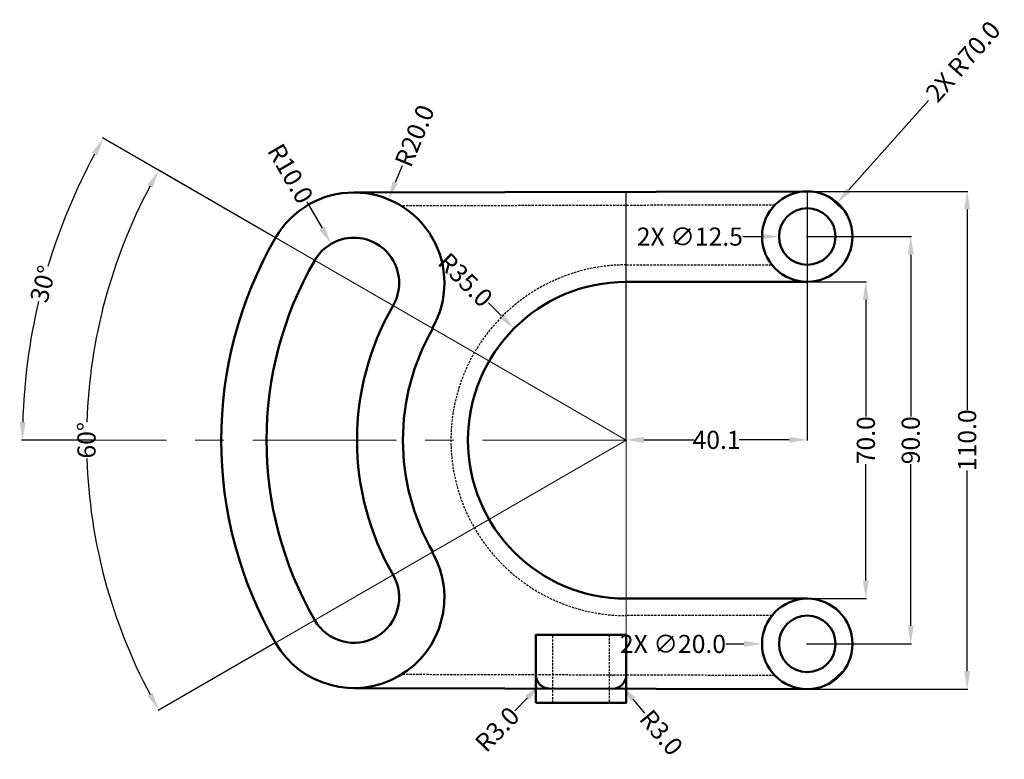
# Model space of a CAD drawing. Units: millimetres. Extents: x 1081 to 1299, y 820 to 983.
import ezdxf

# ---------------------------------------------------------------- set-up
doc = ezdxf.new("R2010")
doc.units = ezdxf.units.MM
doc.header["$MEASUREMENT"] = 0
doc.linetypes.add('CENTER', pattern=[50.8, 31.75, -6.35, 6.35, -6.35])
doc.linetypes.add('HIDDENX2', pattern=[0.75, 0.5, -0.25])
for name, color, linetype, lineweight in [('M-CNTR', 4, 'CENTER', 18), ('M-CONS', 8, 'Continuous', 13), ('M-DIMS', 2, 'Continuous', 25), ('M-HIDN', 3, 'HIDDENX2', 25), ('M-OUTL', 7, 'Continuous', 50)]:
    doc.layers.add(name, color=color, linetype=linetype, lineweight=lineweight)
doc.styles.get("Standard").update_dxf_attribs({"font": 'arial.ttf'})
doc.dimstyles.get("Standard").update_dxf_attribs({"dimtxt": 4, "dimasz": 4, "dimexe": 0.18, "dimexo": 0.0625, "dimgap": 0.09, "dimtad": 0, "dimdec": 1, "dimzin": 0, "dimdsep": 46, "dimtxsty": 'Standard', "dimcen": 0.09, "dimadec": 0, "dimazin": 0, "dimtfac": 1, "dimtdec": 1, "dimtofl": 0, "dimtmove": 0, "dimatfit": 3, "dimfxl": 1, "dimtolj": 1, "dimtzin": 0, "dimarcsym": 0})

# ---------------------------------------------------------------- blocks, each defined once
blk = doc.blocks.new('*D1')
at = {"layer": 'Defpoints', "color": 0, "transparency": 16777216}
for p in [(1137.47, 935.11), (1097.95, 910.82), (1215.42, 890.11), (1215.42, 890.11), (1137.91, 845.36)]:
    blk.add_point(p, dxfattribs=at)
at = {"layer": 'M-DIMS', "color": 0, "lineweight": -2, "transparency": 16777216}
for p, q in [((1137.42, 935.14), (1111.96, 949.84)), ((1137.85, 845.33), (1111.96, 830.38))]:
    blk.add_line(p, q, dxfattribs=at)
for start, end in [(151.9215, 178.0664), (181.9336, 208.0785)]:
    blk.add_arc((1215.42, 890.11), 119.28, start, end, dxfattribs=at)
at = {"layer": 'M-DIMS', "color": 0, "transparency": 16777216}
for points in [[(1109.59, 946.57), (1110.76, 945.93), (1112.12, 949.75)], [(1110.76, 834.29), (1109.59, 833.64), (1112.12, 830.47)]]:
    blk.add_solid(points, dxfattribs=at)
at = {"layer": 'M-DIMS', "color": 0, "transparency": 16777216, "insert": (1096.14, 890.11), "char_height": 4, "attachment_point": 5, "rotation": 90}
blk.add_mtext('\\A1;60°', dxfattribs=at)
blk = doc.blocks.new('*D2')
at = {"layer": 'Defpoints', "color": 0, "transparency": 16777216}
for p in [(1090.03, 935.75), (1137.47, 935.11), (1098.27, 890.11), (1215.42, 890.11), (1215.42, 890.11)]:
    blk.add_point(p, dxfattribs=at)
at = {"layer": 'M-DIMS', "color": 0, "lineweight": -2, "transparency": 16777216}
for p, q in [((1137.42, 935.14), (1099.7, 956.92)), ((1098.21, 890.11), (1081.8, 890.11))]:
    blk.add_line(p, q, dxfattribs=at)
for start, end in [(151.7176, 163.2769), (166.7231, 178.2824)]:
    blk.add_arc((1215.42, 890.11), 133.44, start, end, dxfattribs=at)
at = {"layer": 'M-DIMS', "color": 0, "transparency": 16777216}
for points in [[(1097.33, 953.66), (1098.49, 953.01), (1099.86, 956.83)], [(1082.71, 894.1), (1081.38, 894.12), (1081.98, 890.11)]]:
    blk.add_solid(points, dxfattribs=at)
at = {"layer": 'M-DIMS', "color": 0, "transparency": 16777216, "insert": (1086.53, 924.64), "char_height": 4, "attachment_point": 5, "rotation": 75}
blk.add_mtext('\\A1;30°', dxfattribs=at)
blk = doc.blocks.new('*D3')
at = {"layer": 'Defpoints', "color": 0, "transparency": 16777216}
for p in [(1190.64, 914.82), (1215.42, 890.11)]:
    blk.add_point(p, dxfattribs=at)
at = {"layer": 'M-DIMS', "color": 0, "lineweight": -2, "transparency": 16777216}
for p, q in [((1184.97, 920.47), (1187.8, 917.65)), ((1215.33, 890.11), (1215.51, 890.11)), ((1215.42, 890.02), (1215.42, 890.2))]:
    blk.add_line(p, q, dxfattribs=at)
at = {"layer": 'M-DIMS', "color": 0, "transparency": 16777216}
blk.add_solid([(1188.27, 918.12), (1187.33, 917.18), (1190.64, 914.82)], dxfattribs=at)
at = {"layer": 'M-DIMS', "color": 0, "transparency": 16777216, "insert": (1179.88, 925.55), "char_height": 4, "attachment_point": 5, "rotation": 315.0772}
blk.add_mtext('\\A1;R35.0', dxfattribs=at)
blk = doc.blocks.new('*D4')
at = {"layer": 'Defpoints', "color": 0, "transparency": 16777216}
for p in [(1162.85, 943.35), (1155.23, 924.86)]:
    blk.add_point(p, dxfattribs=at)
at = {"layer": 'M-DIMS', "color": 0, "lineweight": -2, "transparency": 16777216}
for p, q in [((1165.9, 950.74), (1164.38, 947.05)), ((1155.14, 924.86), (1155.32, 924.86)), ((1155.23, 924.77), (1155.23, 924.95))]:
    blk.add_line(p, q, dxfattribs=at)
at = {"layer": 'M-DIMS', "color": 0, "transparency": 16777216}
blk.add_solid([(1163.76, 947.3), (1164.99, 946.79), (1162.85, 943.35)], dxfattribs=at)
at = {"layer": 'M-DIMS', "color": 0, "transparency": 16777216, "insert": (1168.64, 957.39), "char_height": 4, "attachment_point": 5, "rotation": 67.5926}
blk.add_mtext('\\A1;R20.0', dxfattribs=at)
blk = doc.blocks.new('*D5')
at = {"layer": 'Defpoints', "color": 0, "transparency": 16777216}
for p in [(1150.21, 933.51), (1155.23, 924.86)]:
    blk.add_point(p, dxfattribs=at)
at = {"layer": 'M-DIMS', "color": 0, "lineweight": -2, "transparency": 16777216}
for p, q in [((1144.82, 942.8), (1148.2, 936.97)), ((1155.14, 924.86), (1155.32, 924.86)), ((1155.23, 924.77), (1155.23, 924.95))]:
    blk.add_line(p, q, dxfattribs=at)
at = {"layer": 'M-DIMS', "color": 0, "transparency": 16777216}
blk.add_solid([(1148.78, 937.3), (1147.63, 936.63), (1150.21, 933.51)], dxfattribs=at)
at = {"layer": 'M-DIMS', "color": 0, "transparency": 16777216, "insert": (1141.21, 949.03), "char_height": 4, "attachment_point": 5, "rotation": 300.1178}
blk.add_mtext('\\A1;R10.0', dxfattribs=at)
blk = doc.blocks.new('*D6')
at = {"layer": 'Defpoints', "color": 0, "transparency": 16777216}
for p in [(1212.42, 838.22), (1214.36, 835.93)]:
    blk.add_point(p, dxfattribs=at)
at = {"layer": 'M-DIMS', "color": 0, "lineweight": -2, "transparency": 16777216}
for p, q in [((1212.33, 838.22), (1212.51, 838.22)), ((1212.42, 838.13), (1212.42, 838.31)), ((1219.53, 829.82), (1216.94, 832.87))]:
    blk.add_line(p, q, dxfattribs=at)
at = {"layer": 'M-DIMS', "color": 0, "transparency": 16777216}
blk.add_solid([(1217.45, 833.31), (1216.43, 832.44), (1214.36, 835.93)], dxfattribs=at)
at = {"layer": 'M-DIMS', "color": 0, "transparency": 16777216, "insert": (1223.17, 825.52), "char_height": 4, "attachment_point": 5, "rotation": 310.2705}
blk.add_mtext('\\A1;R3.0', dxfattribs=at)
blk = doc.blocks.new('*D7')
at = {"layer": 'Defpoints', "color": 0, "transparency": 16777216}
for p in [(1198.42, 838.25), (1196.34, 836.09)]:
    blk.add_point(p, dxfattribs=at)
at = {"layer": 'M-DIMS', "color": 0, "lineweight": -2, "transparency": 16777216}
for p, q in [((1198.33, 838.25), (1198.51, 838.25)), ((1198.42, 838.16), (1198.42, 838.34)), ((1190.8, 830.31), (1193.57, 833.2))]:
    blk.add_line(p, q, dxfattribs=at)
at = {"layer": 'M-DIMS', "color": 0, "transparency": 16777216}
blk.add_solid([(1193.09, 833.66), (1194.05, 832.74), (1196.34, 836.09)], dxfattribs=at)
at = {"layer": 'M-DIMS', "color": 0, "transparency": 16777216, "insert": (1186.9, 826.24), "char_height": 4, "attachment_point": 5, "rotation": 46.199}
blk.add_mtext('\\A1;R3.0', dxfattribs=at)
blk = doc.blocks.new('*D8')
at = {"layer": 'Defpoints', "color": 0, "transparency": 16777216}
for p in [(1255.42, 935.11), (1255.42, 845.11), (1278.28, 845.11)]:
    blk.add_point(p, dxfattribs=at)
at = {"layer": 'M-DIMS', "color": 0, "lineweight": -2, "transparency": 16777216}
for p, q in [((1255.48, 935.11), (1278.46, 935.11)), ((1278.28, 931.11), (1278.28, 895.39)), ((1278.28, 849.11), (1278.28, 884.83)), ((1255.48, 845.11), (1278.46, 845.11))]:
    blk.add_line(p, q, dxfattribs=at)
at = {"layer": 'M-DIMS', "color": 0, "transparency": 16777216}
for points in [[(1277.61, 931.11), (1278.95, 931.11), (1278.28, 935.11)], [(1277.61, 849.11), (1278.95, 849.11), (1278.28, 845.11)]]:
    blk.add_solid(points, dxfattribs=at)
at = {"layer": 'M-DIMS', "color": 0, "transparency": 16777216, "insert": (1278.28, 890.11), "char_height": 4, "attachment_point": 5, "rotation": 90}
blk.add_mtext('\\A1;90.0', dxfattribs=at)
blk = doc.blocks.new('*D9')
at = {"layer": 'Defpoints', "color": 0, "transparency": 16777216}
for p in [(1255.42, 945.11), (1290.74, 945.11), (1255.42, 835.11)]:
    blk.add_point(p, dxfattribs=at)
at = {"layer": 'M-DIMS', "color": 0, "lineweight": -2, "transparency": 16777216}
for p, q in [((1255.48, 945.11), (1290.92, 945.11)), ((1290.74, 941.11), (1290.74, 896.75)), ((1290.74, 839.11), (1290.74, 883.46)), ((1255.48, 835.11), (1290.92, 835.11))]:
    blk.add_line(p, q, dxfattribs=at)
at = {"layer": 'M-DIMS', "color": 0, "transparency": 16777216}
for points in [[(1290.07, 941.11), (1291.4, 941.11), (1290.74, 945.11)], [(1290.07, 839.11), (1291.4, 839.11), (1290.74, 835.11)]]:
    blk.add_solid(points, dxfattribs=at)
at = {"layer": 'M-DIMS', "color": 0, "transparency": 16777216, "insert": (1290.74, 890.11), "char_height": 4, "attachment_point": 5, "rotation": 90}
blk.add_mtext('\\A1;110.0', dxfattribs=at)
blk = doc.blocks.new('*D10')
at = {"layer": 'Defpoints', "color": 0, "transparency": 16777216}
for p in [(1255.42, 925.11), (1268.36, 925.11), (1255.42, 855.11)]:
    blk.add_point(p, dxfattribs=at)
at = {"layer": 'M-DIMS', "color": 0, "lineweight": -2, "transparency": 16777216}
for p, q in [((1255.48, 925.11), (1268.54, 925.11)), ((1268.36, 921.11), (1268.36, 895.37)), ((1268.36, 859.11), (1268.36, 884.85)), ((1255.48, 855.11), (1268.54, 855.11))]:
    blk.add_line(p, q, dxfattribs=at)
at = {"layer": 'M-DIMS', "color": 0, "transparency": 16777216}
for points in [[(1267.69, 921.11), (1269.03, 921.11), (1268.36, 925.11)], [(1267.69, 859.11), (1269.03, 859.11), (1268.36, 855.11)]]:
    blk.add_solid(points, dxfattribs=at)
at = {"layer": 'M-DIMS', "color": 0, "transparency": 16777216, "insert": (1268.36, 890.11), "char_height": 4, "attachment_point": 5, "rotation": 90}
blk.add_mtext('\\A1;70.0', dxfattribs=at)
blk = doc.blocks.new('*D11')
at = {"layer": 'Defpoints', "color": 0, "transparency": 16777216}
for p in [(1215.33, 945.01), (1255.42, 945.11), (1215.33, 890.2)]:
    blk.add_point(p, dxfattribs=at)
at = {"layer": 'M-DIMS', "color": 0, "lineweight": -2, "transparency": 16777216}
for p, q in [((1215.33, 944.95), (1215.33, 890.02)), ((1255.42, 945.05), (1255.42, 890.02)), ((1219.33, 890.2), (1230.39, 890.2)), ((1251.42, 890.2), (1240.35, 890.2))]:
    blk.add_line(p, q, dxfattribs=at)
at = {"layer": 'M-DIMS', "color": 0, "transparency": 16777216}
for points in [[(1219.33, 890.87), (1219.33, 889.53), (1215.33, 890.2)], [(1251.42, 890.87), (1251.42, 889.53), (1255.42, 890.2)]]:
    blk.add_solid(points, dxfattribs=at)
at = {"layer": 'M-DIMS', "color": 0, "transparency": 16777216, "insert": (1235.37, 890.2), "char_height": 4, "attachment_point": 5}
blk.add_mtext('\\A1;40.1', dxfattribs=at)
blk = doc.blocks.new('MOUNT-TAB-20-BORE-12_5')
for radius in [10, 6.25]:
    blk.add_circle((0, 0), radius)
blk = doc.blocks.new('*D13')
at = {"layer": 'Defpoints', "color": 0, "transparency": 16777216}
for p in [(1261.92, 942.43), (1215.42, 890.11)]:
    blk.add_point(p, dxfattribs=at)
at = {"layer": 'M-DIMS', "color": 0, "lineweight": -2, "transparency": 16777216}
for p, q in [((1282.17, 965.21), (1264.58, 945.42)), ((1215.33, 890.11), (1215.51, 890.11)), ((1215.42, 890.02), (1215.42, 890.2))]:
    blk.add_line(p, q, dxfattribs=at)
at = {"layer": 'M-DIMS', "color": 0, "transparency": 16777216}
blk.add_solid([(1264.08, 945.86), (1265.08, 944.97), (1261.92, 942.43)], dxfattribs=at)
at = {"layer": 'M-DIMS', "color": 0, "transparency": 16777216, "insert": (1289.83, 973.82), "char_height": 4, "attachment_point": 5, "rotation": 48.3661}
blk.add_mtext('\\A1;2X R70.0', dxfattribs=at)
blk = doc.blocks.new('*D14')
at = {"layer": 'Defpoints', "color": 0, "transparency": 16777216}
for p in [(1245.42, 845.11), (1265.42, 845.11)]:
    blk.add_point(p, dxfattribs=at)
at = {"layer": 'M-DIMS', "color": 0, "lineweight": -2, "transparency": 16777216}
for p, q in [((1237.42, 845.11), (1241.42, 845.11)), ((1255.33, 845.11), (1255.51, 845.11)), ((1255.42, 845.02), (1255.42, 845.2))]:
    blk.add_line(p, q, dxfattribs=at)
at = {"layer": 'M-DIMS', "color": 0, "transparency": 16777216}
blk.add_solid([(1241.42, 845.78), (1241.42, 844.44), (1245.42, 845.11)], dxfattribs=at)
at = {"layer": 'M-DIMS', "color": 0, "transparency": 16777216, "insert": (1225.74, 845.11), "char_height": 4, "attachment_point": 5, "rotation": 359.998}
blk.add_mtext('\\A1;2X ∅20.0', dxfattribs=at)
blk = doc.blocks.new('*D15')
at = {"layer": 'Defpoints', "color": 0, "transparency": 16777216}
for p in [(1249.17, 935.11), (1261.67, 935.11)]:
    blk.add_point(p, dxfattribs=at)
at = {"layer": 'M-DIMS', "color": 0, "lineweight": -2, "transparency": 16777216}
for p, q in [((1241.17, 935.11), (1245.17, 935.11)), ((1255.33, 935.11), (1255.51, 935.11)), ((1255.42, 935.02), (1255.42, 935.2))]:
    blk.add_line(p, q, dxfattribs=at)
at = {"layer": 'M-DIMS', "color": 0, "transparency": 16777216}
blk.add_solid([(1245.17, 935.78), (1245.17, 934.44), (1249.17, 935.11)], dxfattribs=at)
at = {"layer": 'M-DIMS', "color": 0, "transparency": 16777216, "insert": (1229.47, 935.11), "char_height": 4, "attachment_point": 5, "rotation": 359.9876}
blk.add_mtext('\\A1;2X ∅12.5', dxfattribs=at)

msp = doc.modelspace()

# ---------------------------------------------------------------- linework, layer by layer
at = {"layer": 'M-CNTR'}
msp.add_line((1215.42, 890.11), (1098.27, 890.11), dxfattribs=at)
at = {"layer": 'M-CONS'}
for p, q in [((1215.42, 890.11), (1137.47, 935.11)), ((1215.42, 925.11), (1215.42, 925.11)), ((1215.42, 890.11), (1137.91, 845.36)), ((1215.42, 890.11), (1215.42, 832.11))]:
    msp.add_line(p, q, dxfattribs=at)
at = {"layer": 'M-HIDN'}
for p, q in [((1248.26, 942.09), (1165.72, 941.88)), ((1215.42, 928.86), (1247.61, 928.86)), ((1247.61, 851.36), (1215.42, 851.36)), ((1199.17, 832.11), (1199.17, 847.11)), ((1211.67, 847.11), (1211.67, 832.11)), ((1248.26, 838.13), (1165.72, 838.33))]:
    msp.add_line(p, q, dxfattribs=at)
msp.add_arc((1215.42, 890.11), 38.75, 90, 270, dxfattribs=at)
at = {"layer": 'M-OUTL'}
for p, q in [((1155.18, 944.86), (1255.39, 945.11)), ((1215.42, 925.11), (1255.42, 925.11)), ((1215.42, 855.11), (1255.42, 855.11)), ((1199.17, 847.11), (1211.67, 847.11)), ((1255.39, 835.11), (1155.18, 835.36)), ((1211.67, 832.11), (1199.17, 832.11))]:
    msp.add_line(p, q, dxfattribs=at)
msp.add_lwpolyline([(1195.42, 832.11), (1195.42, 847.11), (1215.42, 847.11), (1215.42, 832.11)], close=True, dxfattribs=at)
for centre, radius, start, end in [((1155.23, 924.86), 20, 330, 150), ((1215.42, 890.11), 70, 46.5758, 50.1571), ((1215.42, 890.11), 89.5, 150, 210), ((1155.23, 924.86), 10, 330, 150), ((1215.42, 890.11), 79.5, 150, 210), ((1215.42, 890.11), 35, 90, 270), ((1215.42, 890.11), 59.5, 150, 210), ((1215.42, 890.11), 49.36, 150, 210), ((1155.23, 855.36), 20, 210, 30), ((1155.23, 855.36), 10, 210, 30), ((1198.42, 838.25), 3, 180, 269.857), ((1212.42, 838.22), 3, 269.857, 0), ((1215.42, 890.11), 70, 309.8429, 313.4242)]:
    msp.add_arc(centre, radius, start, end, dxfattribs=at)

# ---------------------------------------------------------------- block references
for p in [(1255.42, 935.11), (1255.42, 845.11)]:
    msp.add_blockref('MOUNT-TAB-20-BORE-12_5', p, dxfattribs=at)

# ---------------------------------------------------------------- dimensions: what is measured, and where the dimension line sits
at = {"layer": 'M-DIMS'}
dim = msp.add_radius_dim(center=(1215.42, 890.11), mpoint=(1261.92, 942.43), text='2X <>', dimstyle='Standard', override={"dimdec": 1, "dimlfac": 1, "dimrnd": 0, "dimzin": 0, "dimdsep": 46, "dimlunit": 2}, dxfattribs=at)
dim.commit()
dim.dimension.update_dxf_attribs({"geometry": '*D13', "text_midpoint": (1289.83, 973.82), "dimtype": 164})
for center, mpoint, picture, middle in [((1155.23, 924.86), (1162.85, 943.35), '*D4', (1168.64, 957.39)), ((1215.42, 890.11), (1190.64, 914.82), '*D3', (1179.88, 925.55)), ((1198.42, 838.25), (1196.34, 836.09), '*D7', (1186.9, 826.24)), ((1212.42, 838.22), (1214.36, 835.93), '*D6', (1223.17, 825.52))]:
    dim = msp.add_radius_dim(center=center, mpoint=mpoint, dimstyle='Standard', override={"dimclrd": 0, "dimclre": 0, "dimclrt": 0}, dxfattribs=at)
    dim.commit()
    dim.dimension.update_dxf_attribs({"geometry": picture, "text_midpoint": middle})
for base, line1, picture, middle in [((1090.03, 935.75), ((1215.42, 890.11), (1098.27, 890.11)), '*D2', (1086.53, 924.64)), ((1097.95, 910.82), ((1215.42, 890.11), (1137.91, 845.36)), '*D1', (1096.14, 890.11))]:
    dim = msp.add_angular_dim_2l(base=base, line1=line1, line2=((1215.42, 890.11), (1137.47, 935.11)), dimstyle='Standard', override={"dimclrd": 0, "dimclre": 0, "dimclrt": 0}, dxfattribs=at)
    dim.commit()
    dim.dimension.update_dxf_attribs({"geometry": picture, "text_midpoint": middle})
dim = msp.add_radius_dim(center=(1155.23, 924.86), mpoint=(1150.21, 933.51), dimstyle='Standard', override={"dimclrd": 0, "dimclre": 0, "dimclrt": 0}, dxfattribs=at)
dim.commit()
dim.dimension.update_dxf_attribs({"geometry": '*D5', "text_midpoint": (1141.21, 949.03), "dimtype": 164})
dim = msp.add_linear_dim(base=(1215.33, 890.2), p1=(1255.42, 945.11), p2=(1215.33, 945.01), dimstyle='Standard', override={"dimclrd": 0, "dimclre": 0, "dimclrt": 0}, dxfattribs=at)
dim.commit()
dim.dimension.update_dxf_attribs({"geometry": '*D11', "text_midpoint": (1235.37, 890.2)})
for base, p1, p2, picture, middle in [((1290.74, 945.11), (1255.42, 835.11), (1255.42, 945.11), '*D9', (1290.74, 890.11)), ((1278.28, 845.11), (1255.42, 935.11), (1255.42, 845.11), '*D8', (1278.28, 890.11)), ((1268.36, 925.11), (1255.42, 855.11), (1255.42, 925.11), '*D10', (1268.36, 890.11))]:
    dim = msp.add_linear_dim(base=base, p1=p1, p2=p2, angle=90, dimstyle='Standard', override={"dimclrd": 0, "dimclre": 0, "dimclrt": 0}, dxfattribs=at)
    dim.commit()
    dim.dimension.update_dxf_attribs({"geometry": picture, "text_midpoint": middle})
for p1, p2, picture, middle in [((1261.67, 935.11), (1249.17, 935.11), '*D15', (1229.47, 935.11)), ((1265.42, 845.11), (1245.42, 845.11), '*D14', (1225.74, 845.11))]:
    dim = msp.add_diameter_dim_2p(p1=p1, p2=p2, text='2X <>', dimstyle='Standard', override={"dimdec": 1, "dimlfac": 1, "dimrnd": 0, "dimzin": 0, "dimdsep": 46, "dimlunit": 2}, dxfattribs=at)
    dim.commit()
    dim.dimension.update_dxf_attribs({"geometry": picture, "text_midpoint": middle, "dimtype": 163})

doc.saveas('drawing.dxf')
